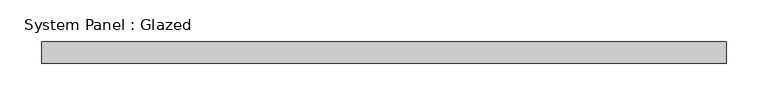
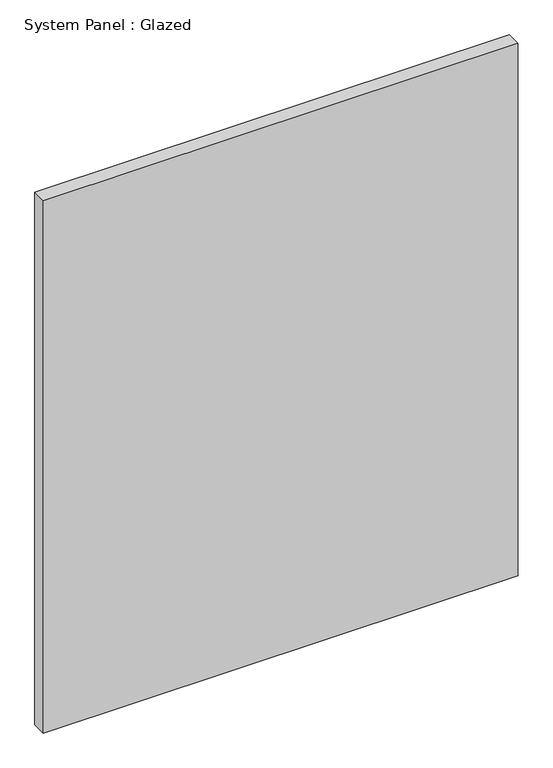
"""IFC4 building model written with IfcOpenShell, lengths in millimetres: plate geometry, System Panel : Glazed."""

from ifc_helpers import new_model, si_unit, origin, origin_with_axes, place, context, project, spatial, polyline, outline, extrude, source, transform, mapped, element, save


def system_panel_glazed_f4fd55f0(model_context):
    return source(origin(), model_context, "Body", "SweptSolid", [
        extrude(outline(polyline([(409.575, 19.05), (-409.575, 19.05), (-409.575, 44.45), (409.575, 44.45), (409.575, 19.05)])), origin_with_axes(), (0.0, 0.0, 1.0), 971.55),
    ])


if __name__ == "__main__":
    model = new_model("IFC4")
    model_context = context("Model", 3, world=origin())
    ifc_project = project(units=[si_unit("LENGTHUNIT", "METRE", prefix="MILLI")], contexts=[model_context])
    site = spatial("IfcSite", under=ifc_project)
    building = spatial("IfcBuilding", under=site)
    placement = place(None, origin())
    system_panel_glazed_shape = system_panel_glazed_f4fd55f0(model_context)
    element("IfcPlate", 1, ObjectType="System Panel : Glazed", at=placement, inside=building, context=model_context, shape_type="MappedRepresentation", body=[
        mapped(system_panel_glazed_shape, transform((0.0, 0.0, 0.0), x_axis=(1.0, 0.0, 0.0), y_axis=(0.0, 1.0, 0.0), z_axis=(0.0, 0.0, 1.0))),
    ])
    save(model, "model.ifc")

# Revit data of these elements
# Type "System Panel : Glazed"
#   Construction Type Id = "GSP4R"
#   Analytic Construction = "1/8 in Pilkington single glazing"
#   Visual Light Transmittance = 0.9
#   Solar Heat Gain Coefficient = 0.86
#   Heat Transfer Coefficient (U) = 1.18115 BTU/(h·ft²·°F)
#   Define Thermal Properties by = 1
# Element 1 (IfcPlate, "System Panel : Glazed")
#   Materials on its faces: "Glass"
# Materials
#   "Glass": class "Glass", colour RGB 0 128 192, transparency 0.75, Description = "Soda Lime Glass", Cost = 0
